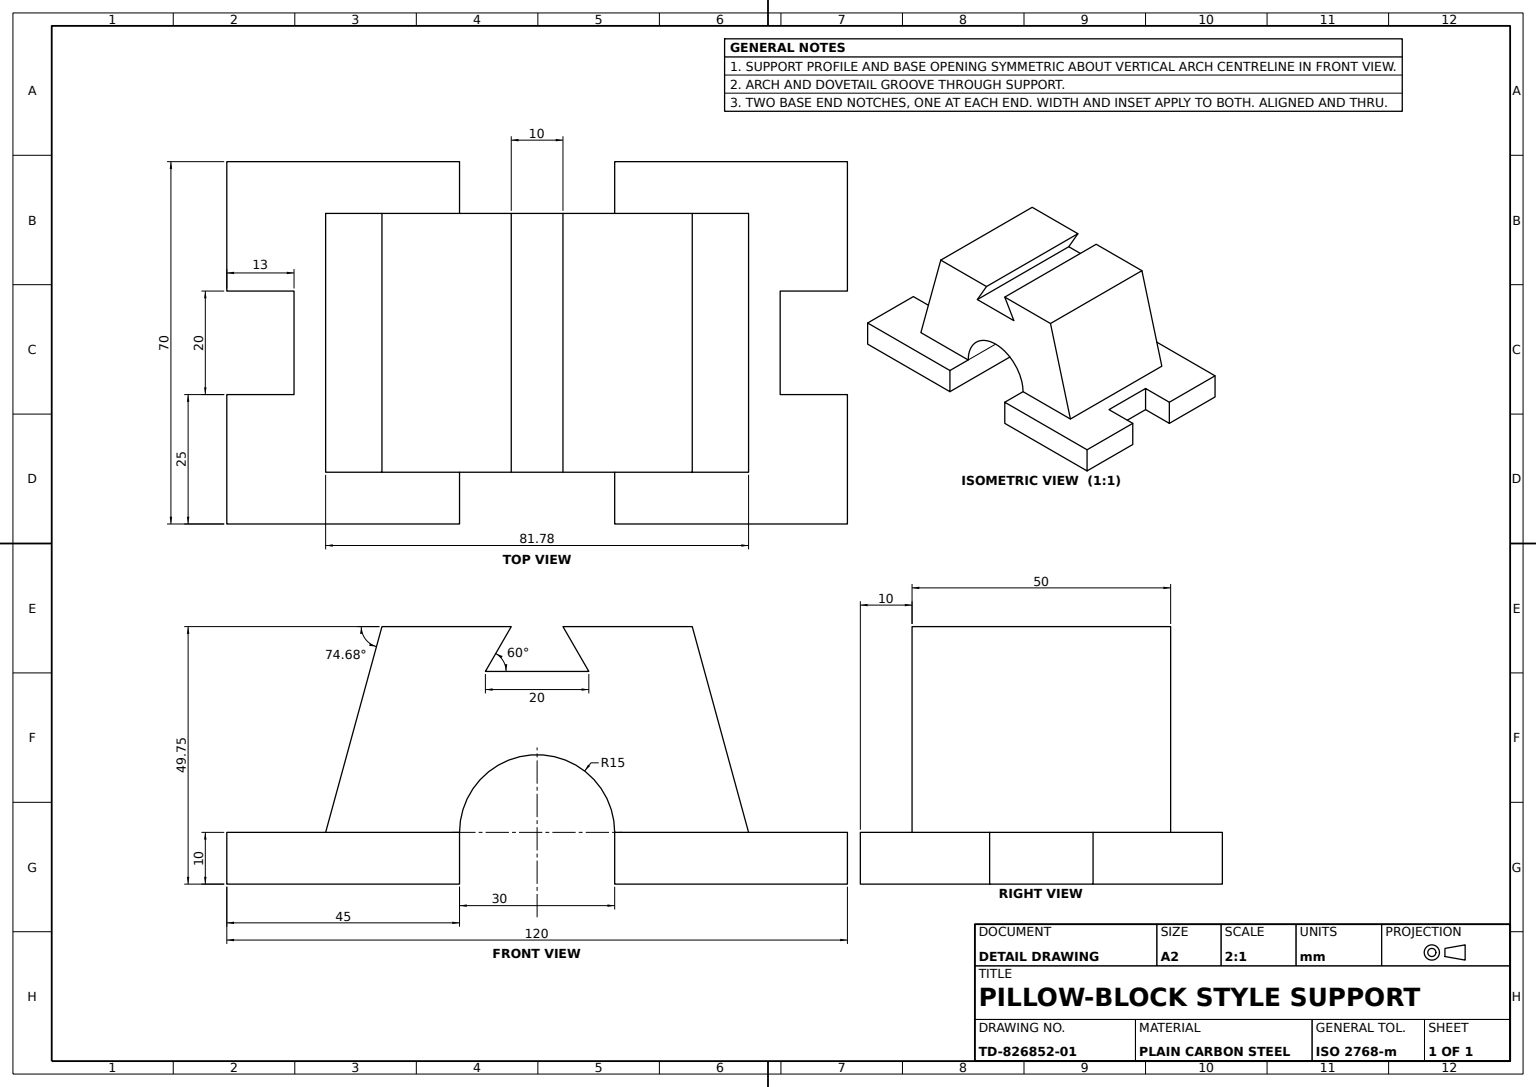
SolidWorks part; units mm, degrees
material "Plain Carbon Steel"
ref_plane "Front Plane" through (0, 0, 0) normal (0, 0, 1) x (1, 0, 0)
ref_plane "Top Plane" through (0, 0, 0) normal (0, 1, 0) x (1, 0, 0)
ref_plane "Right Plane" through (0, 0, 0) normal (1, 0, 0) x (0, 0, -1)
sketch "Base Plate Sketch" plane through (0, 0, 0) normal (0, 1, 0) x (1, 0, 0)
  line L0 (60, 10) -> (42.8083, 10)
  line L1 (-60, -35) -> (60, -35)
  line L2 (-60, -35) -> (-60, -10)
  line L3 (-60, 35) -> (60, 35)
  line L4 (60, -35) -> (60, -10)
  line L5 (-60, -35) -> (60, 35) construction
  line L6 (-60, 35) -> (60, -35) construction
  line L7 (42.8083, 10) -> (42.8083, -10)
  line L8 (42.8083, -10) -> (60, -10)
  line L9 (-60, 10) -> (-44.9851, 10)
  line L10 (-44.9851, 10) -> (-44.9851, -10)
  line L11 (-44.9851, -10) -> (-60, -10)
  line L12 (-60, 10) -> (-60, 35)
  line L13 (60, 10) -> (60, 35)
  point P0 (0, 0)
  dimension "D1" = 120
  dimension "D2" = 70
  dimension "D3" = 25
  dimension "D4" = 25
  dimension "D5" = 25
  dimension "D6" = 25
  dimension "D7" = 20
  dimension "D8" = 42.8083
  dimension "D9" = 44.9851
extrude "Base Plate 10mm" add sketch "Base Plate Sketch" along normal blind 10
sketch "Support Block Profile" plane through (0, 0, 0) normal (0, 0, 1) x (1, 0, 0)
  line L0 (-60, 10) -> (60, 10) construction
  line L1 (-15, 10) -> (-15, 0)
  line L2 (-60, 0) -> (60, 0) construction
  line L3 (15, 10) -> (15, 0)
  line L4 (15, 0) -> (-15, 0)
  line L5 (0, 10) -> (-40.8897, 10)
  line L6 (0, 0) -> (0, 41.0891) construction
  line L7 (-5, 49.7494) -> (-30, 49.7494)
  line L8 (-30, 49.7494) -> (-40.8897, 10)
  line L10 (10, 41.0891) -> (-10, 41.0891)
  line L11 (-10, 41.0891) -> (-5, 49.7494)
  line L12 (0, 41.0891) -> (0, 63.6619) construction
  line L13 (30, 49.7494) -> (40.8897, 10)
  line L14 (10, 41.0891) -> (5, 49.7494)
  line L15 (5, 49.7494) -> (30, 49.7494)
  line L16 (0, 10) -> (40.8897, 10)
  arc A0 (15, 10) -> (-15, 10) centre (0, 10) ccw
  dimension "D1" = 30
  dimension "D2" = 30
  dimension "D3" = 50
  dimension "D4" = 25
  dimension "D5" = 10
  dimension "D6" = 10
  dimension "D7" = 60
  dimension "D8" = 39.7494
  dimension "D9" = 81.7794
extrude "Support Block 50mm" add sketch "Support Block Profile" along normal blind 25 and the other way blind 25 contours A0 L16 L13 L15 L14 L10 L11 L7 L8 L5 | L16 A0 L5
sketch "Arch Cut Sketch" plane through (0, 0, 0) normal (0, 0, 1) x (1, 0, 0)
  line L0 (-40.8897, 10) -> (40.8897, 10) construction
  line L1 (-15, 10) -> (-15, 0)
  line L2 (-60, 0) -> (60, 0) construction
  line L3 (15, 10) -> (15, 0)
  line L4 (15, 0) -> (-15, 0)
  arc A0 (15, 10) -> (-15, 10) centre (0, 10) ccw
  dimension "D1" = 30
  dimension "D2" = 30
extrude "Arch Through Cut" cut sketch "Arch Cut Sketch" against normal blind 35 and the other way blind 35
ref_plane "Boss Plane 44mm" through (-44, 0, 0) normal (1, 0, 0) x (0, 0, -1)
sketch "Upper Boss Sketch" plane through (-44, 0, 0) normal (1, 0, 0) x (0, 0, -1)
  line L0 (-10, 10) -> (10, 10)
  line L1 (25, 10) -> (-25, 10) construction
  line L2 (-10, 10) -> (10, 10) construction
  line L3 (10, 10) -> (10, 0)
  line L4 (10, 0) -> (-10, 0)
  line L5 (-10, 0) -> (-10, 10)
extrude "Upper Boss 3mm" add sketch "Upper Boss Sketch" against normal blind 3
ref_plane "Plane12" through (43, 0, 0) normal (1, 0, 0) x (0, 0, -1)
sketch "Base Pad Sketch" plane through (42.8083, 0, 0) normal (1, 0, 0) x (0, 0, -1)
  line L0 (-10, 10) -> (10, 10)
  line L1 (10, 10) -> (10, 0)
  line L2 (10, 0) -> (-10, 0)
  line L3 (-10, 0) -> (-10, 10)
extrude "Base Pad 4.19mm" add sketch "Base Pad Sketch" along normal blind 4.19
